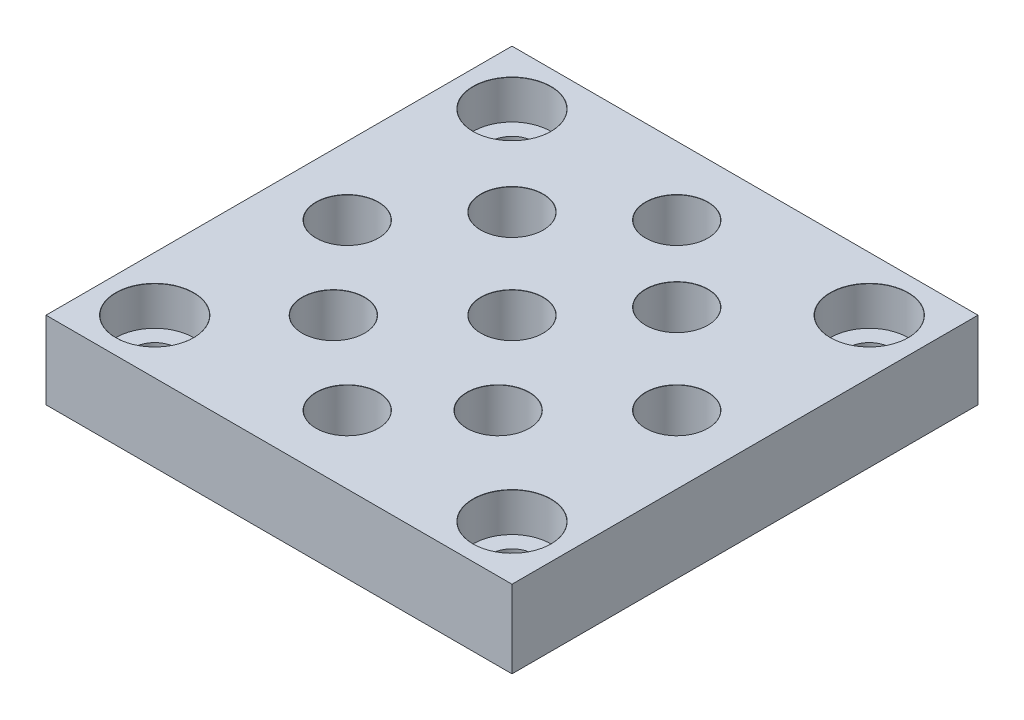
ISO-10303-21;
HEADER;
FILE_DESCRIPTION(('STEP AP214'),'2;1');
FILE_NAME('part.step','',(''),(''),'','','');
FILE_SCHEMA(('AUTOMOTIVE_DESIGN { 1 0 10303 214 1 1 1 1 }'));
ENDSEC;
DATA;
#1=APPLICATION_CONTEXT('core data for automotive mechanical design processes');
#2=APPLICATION_PROTOCOL_DEFINITION('international standard','automotive_design',2000,#1);
#3=PRODUCT_CONTEXT('',#1,'mechanical');
#4=PRODUCT('Part','Part','',(#3));
#5=PRODUCT_RELATED_PRODUCT_CATEGORY('part','',(#4));
#6=PRODUCT_DEFINITION_FORMATION('','',#4);
#7=PRODUCT_DEFINITION_CONTEXT('part definition',#1,'design');
#8=PRODUCT_DEFINITION('design','',#6,#7);
#9=PRODUCT_DEFINITION_SHAPE('','',#8);
#10=(LENGTH_UNIT() NAMED_UNIT(*) SI_UNIT(.MILLI.,.METRE.));
#11=(NAMED_UNIT(*) PLANE_ANGLE_UNIT() SI_UNIT($,.RADIAN.));
#12=(NAMED_UNIT(*) SI_UNIT($,.STERADIAN.) SOLID_ANGLE_UNIT());
#13=UNCERTAINTY_MEASURE_WITH_UNIT(LENGTH_MEASURE(1.E-05),#10,'distance_accuracy_value','');
#14=(GEOMETRIC_REPRESENTATION_CONTEXT(3) GLOBAL_UNCERTAINTY_ASSIGNED_CONTEXT((#13)) GLOBAL_UNIT_ASSIGNED_CONTEXT((#10,
#11,#12)) REPRESENTATION_CONTEXT('',''));
#15=CARTESIAN_POINT('',(0.,0.,0.));
#16=DIRECTION('',(0.,0.,1.));
#17=DIRECTION('',(1.,0.,0.));
#18=AXIS2_PLACEMENT_3D('',#15,#16,#17);
#19=CARTESIAN_POINT('',(0.,10.,0.));
#20=DIRECTION('',(0.,-1.,0.));
#21=DIRECTION('',(0.,0.,-1.));
#22=AXIS2_PLACEMENT_3D('',#19,#20,#21);
#23=PLANE('',#22);
#24=CARTESIAN_POINT('',(-21.2132034355964,10.,0.));
#25=DIRECTION('',(0.,1.,0.));
#26=DIRECTION('',(0.,0.,1.));
#27=AXIS2_PLACEMENT_3D('',#24,#25,#26);
#28=CIRCLE('',#27,4.025);
#29=CARTESIAN_POINT('',(-21.2132034355964,10.,4.025));
#30=VERTEX_POINT('',#29);
#31=EDGE_CURVE('E630',#30,#30,#28,.T.);
#32=ORIENTED_EDGE('',*,*,#31,.F.);
#33=EDGE_LOOP('',(#32));
#34=FACE_BOUND('',#33,.T.);
#35=CARTESIAN_POINT('',(0.,10.,0.));
#36=DIRECTION('',(0.,1.,0.));
#37=DIRECTION('',(0.,0.,1.));
#38=AXIS2_PLACEMENT_3D('',#35,#36,#37);
#39=CIRCLE('',#38,4.025);
#40=CARTESIAN_POINT('',(0.,10.,4.025));
#41=VERTEX_POINT('',#40);
#42=EDGE_CURVE('E176',#41,#41,#39,.T.);
#43=ORIENTED_EDGE('',*,*,#42,.F.);
#44=EDGE_LOOP('',(#43));
#45=FACE_BOUND('',#44,.T.);
#46=CARTESIAN_POINT('',(-11.5,10.,-11.5));
#47=DIRECTION('',(0.,1.,0.));
#48=DIRECTION('',(0.,0.,1.));
#49=AXIS2_PLACEMENT_3D('',#46,#47,#48);
#50=CIRCLE('',#49,4.025);
#51=CARTESIAN_POINT('',(-11.5,10.,-7.475));
#52=VERTEX_POINT('',#51);
#53=EDGE_CURVE('E164',#52,#52,#50,.T.);
#54=ORIENTED_EDGE('',*,*,#53,.F.);
#55=EDGE_LOOP('',(#54));
#56=FACE_BOUND('',#55,.T.);
#57=CARTESIAN_POINT('',(0.,10.,-21.2132034355964));
#58=DIRECTION('',(0.,1.,0.));
#59=DIRECTION('',(0.,0.,1.));
#60=AXIS2_PLACEMENT_3D('',#57,#58,#59);
#61=CIRCLE('',#60,4.025);
#62=CARTESIAN_POINT('',(0.,10.,-17.1882034355964));
#63=VERTEX_POINT('',#62);
#64=EDGE_CURVE('E156',#63,#63,#61,.T.);
#65=ORIENTED_EDGE('',*,*,#64,.F.);
#66=EDGE_LOOP('',(#65));
#67=FACE_BOUND('',#66,.T.);
#68=CARTESIAN_POINT('',(-11.5,10.,11.5));
#69=DIRECTION('',(0.,1.,0.));
#70=DIRECTION('',(0.,0.,1.));
#71=AXIS2_PLACEMENT_3D('',#68,#69,#70);
#72=CIRCLE('',#71,4.025);
#73=CARTESIAN_POINT('',(-11.5,10.,15.525));
#74=VERTEX_POINT('',#73);
#75=EDGE_CURVE('E151',#74,#74,#72,.T.);
#76=ORIENTED_EDGE('',*,*,#75,.F.);
#77=EDGE_LOOP('',(#76));
#78=FACE_BOUND('',#77,.T.);
#79=CARTESIAN_POINT('',(9.71320343559641,10.,11.5));
#80=DIRECTION('',(0.,1.,0.));
#81=DIRECTION('',(0.,0.,1.));
#82=AXIS2_PLACEMENT_3D('',#79,#80,#81);
#83=CIRCLE('',#82,4.025);
#84=CARTESIAN_POINT('',(9.71320343559641,10.,15.525));
#85=VERTEX_POINT('',#84);
#86=EDGE_CURVE('E148',#85,#85,#83,.T.);
#87=ORIENTED_EDGE('',*,*,#86,.F.);
#88=EDGE_LOOP('',(#87));
#89=FACE_BOUND('',#88,.T.);
#90=CARTESIAN_POINT('',(0.,10.,21.2132034355964));
#91=DIRECTION('',(0.,1.,0.));
#92=DIRECTION('',(0.,0.,1.));
#93=AXIS2_PLACEMENT_3D('',#90,#91,#92);
#94=CIRCLE('',#93,4.025);
#95=CARTESIAN_POINT('',(0.,10.,25.2382034355964));
#96=VERTEX_POINT('',#95);
#97=EDGE_CURVE('E143',#96,#96,#94,.T.);
#98=ORIENTED_EDGE('',*,*,#97,.F.);
#99=EDGE_LOOP('',(#98));
#100=FACE_BOUND('',#99,.T.);
#101=CARTESIAN_POINT('',(-23.,10.,-23.));
#102=DIRECTION('',(0.,1.,0.));
#103=DIRECTION('',(0.,0.,1.));
#104=AXIS2_PLACEMENT_3D('',#101,#102,#103);
#105=CIRCLE('',#104,5.025);
#106=CARTESIAN_POINT('',(-23.,10.,-17.975));
#107=VERTEX_POINT('',#106);
#108=EDGE_CURVE('E136',#107,#107,#105,.T.);
#109=ORIENTED_EDGE('',*,*,#108,.F.);
#110=EDGE_LOOP('',(#109));
#111=FACE_BOUND('',#110,.T.);
#112=CARTESIAN_POINT('',(23.,10.,-23.));
#113=DIRECTION('',(0.,1.,0.));
#114=DIRECTION('',(0.,0.,1.));
#115=AXIS2_PLACEMENT_3D('',#112,#113,#114);
#116=CIRCLE('',#115,5.025);
#117=CARTESIAN_POINT('',(23.,10.,-17.975));
#118=VERTEX_POINT('',#117);
#119=EDGE_CURVE('E134',#118,#118,#116,.T.);
#120=ORIENTED_EDGE('',*,*,#119,.F.);
#121=EDGE_LOOP('',(#120));
#122=FACE_BOUND('',#121,.T.);
#123=CARTESIAN_POINT('',(23.,10.,23.));
#124=DIRECTION('',(0.,1.,0.));
#125=DIRECTION('',(0.,0.,1.));
#126=AXIS2_PLACEMENT_3D('',#123,#124,#125);
#127=CIRCLE('',#126,5.025);
#128=CARTESIAN_POINT('',(23.,10.,28.025));
#129=VERTEX_POINT('',#128);
#130=EDGE_CURVE('E127',#129,#129,#127,.T.);
#131=ORIENTED_EDGE('',*,*,#130,.F.);
#132=EDGE_LOOP('',(#131));
#133=FACE_BOUND('',#132,.T.);
#134=CARTESIAN_POINT('',(-23.,10.,23.));
#135=DIRECTION('',(0.,1.,0.));
#136=DIRECTION('',(0.,0.,1.));
#137=AXIS2_PLACEMENT_3D('',#134,#135,#136);
#138=CIRCLE('',#137,5.025);
#139=CARTESIAN_POINT('',(-23.,10.,28.025));
#140=VERTEX_POINT('',#139);
#141=EDGE_CURVE('E121',#140,#140,#138,.T.);
#142=ORIENTED_EDGE('',*,*,#141,.F.);
#143=EDGE_LOOP('',(#142));
#144=FACE_BOUND('',#143,.T.);
#145=DIRECTION('',(0.,0.,1.));
#146=VECTOR('',#145,1.);
#147=CARTESIAN_POINT('',(-30.,10.,-30.));
#148=LINE('',#147,#146);
#149=CARTESIAN_POINT('',(-30.,10.,-30.));
#150=VERTEX_POINT('',#149);
#151=CARTESIAN_POINT('',(-30.,10.,30.));
#152=VERTEX_POINT('',#151);
#153=EDGE_CURVE('E91',#150,#152,#148,.T.);
#154=ORIENTED_EDGE('',*,*,#153,.T.);
#155=DIRECTION('',(1.,0.,0.));
#156=VECTOR('',#155,1.);
#157=CARTESIAN_POINT('',(30.,10.,30.));
#158=LINE('',#157,#156);
#159=CARTESIAN_POINT('',(30.,10.,30.));
#160=VERTEX_POINT('',#159);
#161=EDGE_CURVE('E86',#152,#160,#158,.T.);
#162=ORIENTED_EDGE('',*,*,#161,.T.);
#163=DIRECTION('',(0.,0.,-1.));
#164=VECTOR('',#163,1.);
#165=CARTESIAN_POINT('',(30.,10.,-30.));
#166=LINE('',#165,#164);
#167=CARTESIAN_POINT('',(30.,10.,-30.));
#168=VERTEX_POINT('',#167);
#169=EDGE_CURVE('E93',#160,#168,#166,.T.);
#170=ORIENTED_EDGE('',*,*,#169,.T.);
#171=DIRECTION('',(-1.,0.,0.));
#172=VECTOR('',#171,1.);
#173=CARTESIAN_POINT('',(30.,10.,-30.));
#174=LINE('',#173,#172);
#175=EDGE_CURVE('E59',#168,#150,#174,.T.);
#176=ORIENTED_EDGE('',*,*,#175,.T.);
#177=EDGE_LOOP('',(#154,#162,#170,#176));
#178=FACE_BOUND('',#177,.T.);
#179=CARTESIAN_POINT('',(9.71320343559641,10.,-11.5));
#180=DIRECTION('',(0.,1.,0.));
#181=DIRECTION('',(0.,0.,1.));
#182=AXIS2_PLACEMENT_3D('',#179,#180,#181);
#183=CIRCLE('',#182,4.025);
#184=CARTESIAN_POINT('',(9.71320343559641,10.,-7.475));
#185=VERTEX_POINT('',#184);
#186=EDGE_CURVE('E161',#185,#185,#183,.T.);
#187=ORIENTED_EDGE('',*,*,#186,.F.);
#188=EDGE_LOOP('',(#187));
#189=FACE_BOUND('',#188,.T.);
#190=CARTESIAN_POINT('',(21.2132034355964,10.,0.));
#191=DIRECTION('',(0.,1.,0.));
#192=DIRECTION('',(0.,0.,1.));
#193=AXIS2_PLACEMENT_3D('',#190,#191,#192);
#194=CIRCLE('',#193,4.025);
#195=CARTESIAN_POINT('',(21.2132034355964,10.,4.025));
#196=VERTEX_POINT('',#195);
#197=EDGE_CURVE('E166',#196,#196,#194,.T.);
#198=ORIENTED_EDGE('',*,*,#197,.F.);
#199=EDGE_LOOP('',(#198));
#200=FACE_BOUND('',#199,.T.);
#201=ADVANCED_FACE('F39',(#34,#45,#56,#67,#78,#89,#100,#111,#122,#133,#144,#178,#189,#200),#23,.F.);
#202=CARTESIAN_POINT('',(-30.,10.,-30.));
#203=DIRECTION('',(1.,0.,0.));
#204=DIRECTION('',(0.,0.,-1.));
#205=AXIS2_PLACEMENT_3D('',#202,#203,#204);
#206=PLANE('',#205);
#207=DIRECTION('',(0.,0.,1.));
#208=VECTOR('',#207,1.);
#209=CARTESIAN_POINT('',(-30.,0.,-30.));
#210=LINE('',#209,#208);
#211=CARTESIAN_POINT('',(-30.,0.,-30.));
#212=VERTEX_POINT('',#211);
#213=CARTESIAN_POINT('',(-30.,0.,30.));
#214=VERTEX_POINT('',#213);
#215=EDGE_CURVE('E106',#212,#214,#210,.T.);
#216=ORIENTED_EDGE('',*,*,#215,.T.);
#217=DIRECTION('',(0.,-1.,0.));
#218=VECTOR('',#217,1.);
#219=CARTESIAN_POINT('',(-30.,10.,30.));
#220=LINE('',#219,#218);
#221=EDGE_CURVE('E11',#152,#214,#220,.T.);
#222=ORIENTED_EDGE('',*,*,#221,.F.);
#223=ORIENTED_EDGE('',*,*,#153,.F.);
#224=DIRECTION('',(0.,-1.,0.));
#225=VECTOR('',#224,1.);
#226=CARTESIAN_POINT('',(-30.,10.,-30.));
#227=LINE('',#226,#225);
#228=EDGE_CURVE('E105',#150,#212,#227,.T.);
#229=ORIENTED_EDGE('',*,*,#228,.T.);
#230=EDGE_LOOP('',(#216,#222,#223,#229));
#231=FACE_BOUND('',#230,.T.);
#232=ADVANCED_FACE('F41',(#231),#206,.F.);
#233=CARTESIAN_POINT('',(30.,10.,30.));
#234=DIRECTION('',(0.,0.,-1.));
#235=DIRECTION('',(-1.,0.,0.));
#236=AXIS2_PLACEMENT_3D('',#233,#234,#235);
#237=PLANE('',#236);
#238=DIRECTION('',(1.,0.,0.));
#239=VECTOR('',#238,1.);
#240=CARTESIAN_POINT('',(30.,0.,30.));
#241=LINE('',#240,#239);
#242=CARTESIAN_POINT('',(30.,0.,30.));
#243=VERTEX_POINT('',#242);
#244=EDGE_CURVE('E100',#214,#243,#241,.T.);
#245=ORIENTED_EDGE('',*,*,#244,.T.);
#246=DIRECTION('',(0.,-1.,0.));
#247=VECTOR('',#246,1.);
#248=CARTESIAN_POINT('',(30.,10.,30.));
#249=LINE('',#248,#247);
#250=EDGE_CURVE('E47',#160,#243,#249,.T.);
#251=ORIENTED_EDGE('',*,*,#250,.F.);
#252=ORIENTED_EDGE('',*,*,#161,.F.);
#253=ORIENTED_EDGE('',*,*,#221,.T.);
#254=EDGE_LOOP('',(#245,#251,#252,#253));
#255=FACE_BOUND('',#254,.T.);
#256=ADVANCED_FACE('F96',(#255),#237,.F.);
#257=CARTESIAN_POINT('',(30.,10.,-30.));
#258=DIRECTION('',(-1.,0.,0.));
#259=DIRECTION('',(0.,0.,1.));
#260=AXIS2_PLACEMENT_3D('',#257,#258,#259);
#261=PLANE('',#260);
#262=DIRECTION('',(0.,0.,-1.));
#263=VECTOR('',#262,1.);
#264=CARTESIAN_POINT('',(30.,0.,-30.));
#265=LINE('',#264,#263);
#266=CARTESIAN_POINT('',(30.,0.,-30.));
#267=VERTEX_POINT('',#266);
#268=EDGE_CURVE('E73',#243,#267,#265,.T.);
#269=ORIENTED_EDGE('',*,*,#268,.T.);
#270=DIRECTION('',(0.,-1.,0.));
#271=VECTOR('',#270,1.);
#272=CARTESIAN_POINT('',(30.,10.,-30.));
#273=LINE('',#272,#271);
#274=EDGE_CURVE('E98',#168,#267,#273,.T.);
#275=ORIENTED_EDGE('',*,*,#274,.F.);
#276=ORIENTED_EDGE('',*,*,#169,.F.);
#277=ORIENTED_EDGE('',*,*,#250,.T.);
#278=EDGE_LOOP('',(#269,#275,#276,#277));
#279=FACE_BOUND('',#278,.T.);
#280=ADVANCED_FACE('F99',(#279),#261,.F.);
#281=CARTESIAN_POINT('',(30.,10.,-30.));
#282=DIRECTION('',(0.,0.,1.));
#283=DIRECTION('',(1.,0.,0.));
#284=AXIS2_PLACEMENT_3D('',#281,#282,#283);
#285=PLANE('',#284);
#286=DIRECTION('',(-1.,0.,0.));
#287=VECTOR('',#286,1.);
#288=CARTESIAN_POINT('',(30.,0.,-30.));
#289=LINE('',#288,#287);
#290=EDGE_CURVE('E81',#267,#212,#289,.T.);
#291=ORIENTED_EDGE('',*,*,#290,.T.);
#292=ORIENTED_EDGE('',*,*,#228,.F.);
#293=ORIENTED_EDGE('',*,*,#175,.F.);
#294=ORIENTED_EDGE('',*,*,#274,.T.);
#295=EDGE_LOOP('',(#291,#292,#293,#294));
#296=FACE_BOUND('',#295,.T.);
#297=ADVANCED_FACE('F290',(#296),#285,.F.);
#298=CARTESIAN_POINT('',(0.,0.,0.));
#299=DIRECTION('',(0.,-1.,0.));
#300=DIRECTION('',(0.,0.,-1.));
#301=AXIS2_PLACEMENT_3D('',#298,#299,#300);
#302=PLANE('',#301);
#303=CARTESIAN_POINT('',(-21.2132034355964,0.,0.));
#304=DIRECTION('',(0.,-1.,0.));
#305=DIRECTION('',(0.,0.,-1.));
#306=AXIS2_PLACEMENT_3D('',#303,#304,#305);
#307=CIRCLE('',#306,3.99999999999999);
#308=CARTESIAN_POINT('',(-21.2132034355964,0.,-4.));
#309=VERTEX_POINT('',#308);
#310=EDGE_CURVE('E43',#309,#309,#307,.T.);
#311=ORIENTED_EDGE('',*,*,#310,.F.);
#312=EDGE_LOOP('',(#311));
#313=FACE_BOUND('',#312,.T.);
#314=CARTESIAN_POINT('',(0.,0.,0.));
#315=DIRECTION('',(0.,-1.,0.));
#316=DIRECTION('',(0.,0.,-1.));
#317=AXIS2_PLACEMENT_3D('',#314,#315,#316);
#318=CIRCLE('',#317,3.99999999999999);
#319=CARTESIAN_POINT('',(0.,0.,-3.99999999999999));
#320=VERTEX_POINT('',#319);
#321=EDGE_CURVE('E170',#320,#320,#318,.T.);
#322=ORIENTED_EDGE('',*,*,#321,.F.);
#323=EDGE_LOOP('',(#322));
#324=FACE_BOUND('',#323,.T.);
#325=CARTESIAN_POINT('',(21.2132034355964,0.,0.));
#326=DIRECTION('',(0.,-1.,0.));
#327=DIRECTION('',(0.,0.,-1.));
#328=AXIS2_PLACEMENT_3D('',#325,#326,#327);
#329=CIRCLE('',#328,3.99999999999999);
#330=CARTESIAN_POINT('',(21.2132034355964,0.,-3.99999999999999));
#331=VERTEX_POINT('',#330);
#332=EDGE_CURVE('E162',#331,#331,#329,.T.);
#333=ORIENTED_EDGE('',*,*,#332,.F.);
#334=EDGE_LOOP('',(#333));
#335=FACE_BOUND('',#334,.T.);
#336=CARTESIAN_POINT('',(-11.5,0.,-11.5));
#337=DIRECTION('',(0.,-1.,0.));
#338=DIRECTION('',(0.,0.,-1.));
#339=AXIS2_PLACEMENT_3D('',#336,#337,#338);
#340=CIRCLE('',#339,3.99999999999999);
#341=CARTESIAN_POINT('',(-11.5,0.,-15.5));
#342=VERTEX_POINT('',#341);
#343=EDGE_CURVE('E158',#342,#342,#340,.T.);
#344=ORIENTED_EDGE('',*,*,#343,.F.);
#345=EDGE_LOOP('',(#344));
#346=FACE_BOUND('',#345,.T.);
#347=CARTESIAN_POINT('',(9.71320343559641,0.,-11.5));
#348=DIRECTION('',(0.,-1.,0.));
#349=DIRECTION('',(0.,0.,-1.));
#350=AXIS2_PLACEMENT_3D('',#347,#348,#349);
#351=CIRCLE('',#350,3.99999999999999);
#352=CARTESIAN_POINT('',(9.71320343559641,0.,-15.5));
#353=VERTEX_POINT('',#352);
#354=EDGE_CURVE('E153',#353,#353,#351,.T.);
#355=ORIENTED_EDGE('',*,*,#354,.F.);
#356=EDGE_LOOP('',(#355));
#357=FACE_BOUND('',#356,.T.);
#358=CARTESIAN_POINT('',(0.,0.,-21.2132034355964));
#359=DIRECTION('',(0.,-1.,0.));
#360=DIRECTION('',(0.,0.,-1.));
#361=AXIS2_PLACEMENT_3D('',#358,#359,#360);
#362=CIRCLE('',#361,3.99999999999999);
#363=CARTESIAN_POINT('',(0.,0.,-25.2132034355964));
#364=VERTEX_POINT('',#363);
#365=EDGE_CURVE('E146',#364,#364,#362,.T.);
#366=ORIENTED_EDGE('',*,*,#365,.F.);
#367=EDGE_LOOP('',(#366));
#368=FACE_BOUND('',#367,.T.);
#369=CARTESIAN_POINT('',(-11.5,0.,11.5));
#370=DIRECTION('',(0.,-1.,0.));
#371=DIRECTION('',(0.,0.,-1.));
#372=AXIS2_PLACEMENT_3D('',#369,#370,#371);
#373=CIRCLE('',#372,3.99999999999999);
#374=CARTESIAN_POINT('',(-11.5,0.,7.5));
#375=VERTEX_POINT('',#374);
#376=EDGE_CURVE('E141',#375,#375,#373,.T.);
#377=ORIENTED_EDGE('',*,*,#376,.F.);
#378=EDGE_LOOP('',(#377));
#379=FACE_BOUND('',#378,.T.);
#380=CARTESIAN_POINT('',(9.71320343559641,0.,11.5));
#381=DIRECTION('',(0.,-1.,0.));
#382=DIRECTION('',(0.,0.,-1.));
#383=AXIS2_PLACEMENT_3D('',#380,#381,#382);
#384=CIRCLE('',#383,3.99999999999999);
#385=CARTESIAN_POINT('',(9.71320343559641,0.,7.50000000000001));
#386=VERTEX_POINT('',#385);
#387=EDGE_CURVE('E138',#386,#386,#384,.T.);
#388=ORIENTED_EDGE('',*,*,#387,.F.);
#389=EDGE_LOOP('',(#388));
#390=FACE_BOUND('',#389,.T.);
#391=CARTESIAN_POINT('',(0.,0.,21.2132034355964));
#392=DIRECTION('',(0.,-1.,0.));
#393=DIRECTION('',(0.,0.,-1.));
#394=AXIS2_PLACEMENT_3D('',#391,#392,#393);
#395=CIRCLE('',#394,3.99999999999999);
#396=CARTESIAN_POINT('',(0.,0.,17.2132034355964));
#397=VERTEX_POINT('',#396);
#398=EDGE_CURVE('E135',#397,#397,#395,.T.);
#399=ORIENTED_EDGE('',*,*,#398,.F.);
#400=EDGE_LOOP('',(#399));
#401=FACE_BOUND('',#400,.T.);
#402=CARTESIAN_POINT('',(-23.,0.,-23.));
#403=DIRECTION('',(0.,-1.,0.));
#404=DIRECTION('',(0.,0.,-1.));
#405=AXIS2_PLACEMENT_3D('',#402,#403,#404);
#406=CIRCLE('',#405,2.74999999999999);
#407=CARTESIAN_POINT('',(-23.,0.,-25.75));
#408=VERTEX_POINT('',#407);
#409=EDGE_CURVE('E126',#408,#408,#406,.T.);
#410=ORIENTED_EDGE('',*,*,#409,.F.);
#411=EDGE_LOOP('',(#410));
#412=FACE_BOUND('',#411,.T.);
#413=CARTESIAN_POINT('',(23.,0.,-23.));
#414=DIRECTION('',(0.,-1.,0.));
#415=DIRECTION('',(0.,0.,-1.));
#416=AXIS2_PLACEMENT_3D('',#413,#414,#415);
#417=CIRCLE('',#416,2.74999999999999);
#418=CARTESIAN_POINT('',(23.,0.,-25.75));
#419=VERTEX_POINT('',#418);
#420=EDGE_CURVE('E123',#419,#419,#417,.T.);
#421=ORIENTED_EDGE('',*,*,#420,.F.);
#422=EDGE_LOOP('',(#421));
#423=FACE_BOUND('',#422,.T.);
#424=CARTESIAN_POINT('',(23.,0.,23.));
#425=DIRECTION('',(0.,-1.,0.));
#426=DIRECTION('',(0.,0.,-1.));
#427=AXIS2_PLACEMENT_3D('',#424,#425,#426);
#428=CIRCLE('',#427,2.74999999999999);
#429=CARTESIAN_POINT('',(23.,0.,20.25));
#430=VERTEX_POINT('',#429);
#431=EDGE_CURVE('E120',#430,#430,#428,.T.);
#432=ORIENTED_EDGE('',*,*,#431,.F.);
#433=EDGE_LOOP('',(#432));
#434=FACE_BOUND('',#433,.T.);
#435=CARTESIAN_POINT('',(-23.,0.,23.));
#436=DIRECTION('',(0.,-1.,0.));
#437=DIRECTION('',(0.,0.,-1.));
#438=AXIS2_PLACEMENT_3D('',#435,#436,#437);
#439=CIRCLE('',#438,2.74999999999999);
#440=CARTESIAN_POINT('',(-23.,0.,20.25));
#441=VERTEX_POINT('',#440);
#442=EDGE_CURVE('E108',#441,#441,#439,.T.);
#443=ORIENTED_EDGE('',*,*,#442,.F.);
#444=EDGE_LOOP('',(#443));
#445=FACE_BOUND('',#444,.T.);
#446=ORIENTED_EDGE('',*,*,#215,.F.);
#447=ORIENTED_EDGE('',*,*,#290,.F.);
#448=ORIENTED_EDGE('',*,*,#268,.F.);
#449=ORIENTED_EDGE('',*,*,#244,.F.);
#450=EDGE_LOOP('',(#446,#447,#448,#449));
#451=FACE_BOUND('',#450,.T.);
#452=ADVANCED_FACE('F282',(#313,#324,#335,#346,#357,#368,#379,#390,#401,#412,#423,#434,#445,
#451),#302,.T.);
#453=CARTESIAN_POINT('',(-23.,10.,23.));
#454=DIRECTION('',(0.,1.,0.));
#455=DIRECTION('',(0.,0.,1.));
#456=AXIS2_PLACEMENT_3D('',#453,#454,#455);
#457=CYLINDRICAL_SURFACE('',#456,2.74999999999999);
#458=ORIENTED_EDGE('',*,*,#442,.T.);
#459=EDGE_LOOP('',(#458));
#460=FACE_BOUND('',#459,.T.);
#461=CARTESIAN_POINT('',(-23.,5.,23.));
#462=DIRECTION('',(0.,1.,0.));
#463=DIRECTION('',(0.,0.,1.));
#464=AXIS2_PLACEMENT_3D('',#461,#462,#463);
#465=CIRCLE('',#464,2.75);
#466=CARTESIAN_POINT('',(-23.,5.,25.75));
#467=VERTEX_POINT('',#466);
#468=EDGE_CURVE('E116',#467,#467,#465,.T.);
#469=ORIENTED_EDGE('',*,*,#468,.T.);
#470=EDGE_LOOP('',(#469));
#471=FACE_BOUND('',#470,.T.);
#472=ADVANCED_FACE('F253',(#460,#471),#457,.F.);
#473=CARTESIAN_POINT('',(-20.25,5.,23.));
#474=DIRECTION('',(0.,-1.,0.));
#475=DIRECTION('',(0.,0.,-1.));
#476=AXIS2_PLACEMENT_3D('',#473,#474,#475);
#477=PLANE('',#476);
#478=ORIENTED_EDGE('',*,*,#468,.F.);
#479=EDGE_LOOP('',(#478));
#480=FACE_BOUND('',#479,.T.);
#481=CARTESIAN_POINT('',(-23.,5.,23.));
#482=DIRECTION('',(0.,1.,0.));
#483=DIRECTION('',(0.,0.,1.));
#484=AXIS2_PLACEMENT_3D('',#481,#482,#483);
#485=CIRCLE('',#484,5.);
#486=CARTESIAN_POINT('',(-23.,5.,28.));
#487=VERTEX_POINT('',#486);
#488=EDGE_CURVE('E242',#487,#487,#485,.T.);
#489=ORIENTED_EDGE('',*,*,#488,.T.);
#490=EDGE_LOOP('',(#489));
#491=FACE_BOUND('',#490,.T.);
#492=ADVANCED_FACE('F251',(#480,#491),#477,.F.);
#493=CARTESIAN_POINT('',(-23.,10.,23.));
#494=DIRECTION('',(0.,1.,0.));
#495=DIRECTION('',(0.,0.,1.));
#496=AXIS2_PLACEMENT_3D('',#493,#494,#495);
#497=CYLINDRICAL_SURFACE('',#496,5.);
#498=ORIENTED_EDGE('',*,*,#488,.F.);
#499=EDGE_LOOP('',(#498));
#500=FACE_BOUND('',#499,.T.);
#501=CARTESIAN_POINT('',(-23.,9.97902250922057,23.));
#502=DIRECTION('',(0.,1.,0.));
#503=DIRECTION('',(0.,0.,1.));
#504=AXIS2_PLACEMENT_3D('',#501,#502,#503);
#505=CIRCLE('',#504,5.);
#506=CARTESIAN_POINT('',(-23.,9.97902250922057,28.));
#507=VERTEX_POINT('',#506);
#508=EDGE_CURVE('E241',#507,#507,#505,.T.);
#509=ORIENTED_EDGE('',*,*,#508,.T.);
#510=EDGE_LOOP('',(#509));
#511=FACE_BOUND('',#510,.T.);
#512=ADVANCED_FACE('F258',(#500,#511),#497,.F.);
#513=CARTESIAN_POINT('',(-23.,10.,23.));
#514=DIRECTION('',(0.,1.,0.));
#515=DIRECTION('',(0.,0.,1.));
#516=AXIS2_PLACEMENT_3D('',#513,#514,#515);
#517=CONICAL_SURFACE('',#516,5.025,0.872664625997159);
#518=ORIENTED_EDGE('',*,*,#508,.F.);
#519=EDGE_LOOP('',(#518));
#520=FACE_BOUND('',#519,.T.);
#521=ORIENTED_EDGE('',*,*,#141,.T.);
#522=EDGE_LOOP('',(#521));
#523=FACE_BOUND('',#522,.T.);
#524=ADVANCED_FACE('F265',(#520,#523),#517,.F.);
#525=CARTESIAN_POINT('',(23.,10.,23.));
#526=DIRECTION('',(0.,1.,0.));
#527=DIRECTION('',(0.,0.,1.));
#528=AXIS2_PLACEMENT_3D('',#525,#526,#527);
#529=CYLINDRICAL_SURFACE('',#528,2.74999999999999);
#530=ORIENTED_EDGE('',*,*,#431,.T.);
#531=EDGE_LOOP('',(#530));
#532=FACE_BOUND('',#531,.T.);
#533=CARTESIAN_POINT('',(23.,5.,23.));
#534=DIRECTION('',(0.,1.,0.));
#535=DIRECTION('',(0.,0.,1.));
#536=AXIS2_PLACEMENT_3D('',#533,#534,#535);
#537=CIRCLE('',#536,2.75);
#538=CARTESIAN_POINT('',(23.,5.,25.75));
#539=VERTEX_POINT('',#538);
#540=EDGE_CURVE('E125',#539,#539,#537,.T.);
#541=ORIENTED_EDGE('',*,*,#540,.T.);
#542=EDGE_LOOP('',(#541));
#543=FACE_BOUND('',#542,.T.);
#544=ADVANCED_FACE('F268',(#532,#543),#529,.F.);
#545=CARTESIAN_POINT('',(25.75,5.,23.));
#546=DIRECTION('',(0.,-1.,0.));
#547=DIRECTION('',(0.,0.,-1.));
#548=AXIS2_PLACEMENT_3D('',#545,#546,#547);
#549=PLANE('',#548);
#550=ORIENTED_EDGE('',*,*,#540,.F.);
#551=EDGE_LOOP('',(#550));
#552=FACE_BOUND('',#551,.T.);
#553=CARTESIAN_POINT('',(23.,5.,23.));
#554=DIRECTION('',(0.,1.,0.));
#555=DIRECTION('',(0.,0.,1.));
#556=AXIS2_PLACEMENT_3D('',#553,#554,#555);
#557=CIRCLE('',#556,5.);
#558=CARTESIAN_POINT('',(23.,5.,28.));
#559=VERTEX_POINT('',#558);
#560=EDGE_CURVE('E234',#559,#559,#557,.T.);
#561=ORIENTED_EDGE('',*,*,#560,.T.);
#562=EDGE_LOOP('',(#561));
#563=FACE_BOUND('',#562,.T.);
#564=ADVANCED_FACE('F336',(#552,#563),#549,.F.);
#565=CARTESIAN_POINT('',(23.,10.,23.));
#566=DIRECTION('',(0.,1.,0.));
#567=DIRECTION('',(0.,0.,1.));
#568=AXIS2_PLACEMENT_3D('',#565,#566,#567);
#569=CYLINDRICAL_SURFACE('',#568,5.);
#570=ORIENTED_EDGE('',*,*,#560,.F.);
#571=EDGE_LOOP('',(#570));
#572=FACE_BOUND('',#571,.T.);
#573=CARTESIAN_POINT('',(23.,9.97902250922057,23.));
#574=DIRECTION('',(0.,1.,0.));
#575=DIRECTION('',(0.,0.,1.));
#576=AXIS2_PLACEMENT_3D('',#573,#574,#575);
#577=CIRCLE('',#576,5.);
#578=CARTESIAN_POINT('',(23.,9.97902250922057,28.));
#579=VERTEX_POINT('',#578);
#580=EDGE_CURVE('E235',#579,#579,#577,.T.);
#581=ORIENTED_EDGE('',*,*,#580,.T.);
#582=EDGE_LOOP('',(#581));
#583=FACE_BOUND('',#582,.T.);
#584=ADVANCED_FACE('F347',(#572,#583),#569,.F.);
#585=CARTESIAN_POINT('',(23.,10.,23.));
#586=DIRECTION('',(0.,1.,0.));
#587=DIRECTION('',(0.,0.,1.));
#588=AXIS2_PLACEMENT_3D('',#585,#586,#587);
#589=CONICAL_SURFACE('',#588,5.025,0.872664625997159);
#590=ORIENTED_EDGE('',*,*,#580,.F.);
#591=EDGE_LOOP('',(#590));
#592=FACE_BOUND('',#591,.T.);
#593=ORIENTED_EDGE('',*,*,#130,.T.);
#594=EDGE_LOOP('',(#593));
#595=FACE_BOUND('',#594,.T.);
#596=ADVANCED_FACE('F352',(#592,#595),#589,.F.);
#597=CARTESIAN_POINT('',(23.,10.,-23.));
#598=DIRECTION('',(0.,1.,0.));
#599=DIRECTION('',(0.,0.,1.));
#600=AXIS2_PLACEMENT_3D('',#597,#598,#599);
#601=CYLINDRICAL_SURFACE('',#600,2.74999999999999);
#602=ORIENTED_EDGE('',*,*,#420,.T.);
#603=EDGE_LOOP('',(#602));
#604=FACE_BOUND('',#603,.T.);
#605=CARTESIAN_POINT('',(23.,5.,-23.));
#606=DIRECTION('',(0.,1.,0.));
#607=DIRECTION('',(0.,0.,1.));
#608=AXIS2_PLACEMENT_3D('',#605,#606,#607);
#609=CIRCLE('',#608,2.75);
#610=CARTESIAN_POINT('',(23.,5.,-20.25));
#611=VERTEX_POINT('',#610);
#612=EDGE_CURVE('E130',#611,#611,#609,.T.);
#613=ORIENTED_EDGE('',*,*,#612,.T.);
#614=EDGE_LOOP('',(#613));
#615=FACE_BOUND('',#614,.T.);
#616=ADVANCED_FACE('F365',(#604,#615),#601,.F.);
#617=CARTESIAN_POINT('',(25.75,5.,-23.));
#618=DIRECTION('',(0.,-1.,0.));
#619=DIRECTION('',(0.,0.,-1.));
#620=AXIS2_PLACEMENT_3D('',#617,#618,#619);
#621=PLANE('',#620);
#622=ORIENTED_EDGE('',*,*,#612,.F.);
#623=EDGE_LOOP('',(#622));
#624=FACE_BOUND('',#623,.T.);
#625=CARTESIAN_POINT('',(23.,5.,-23.));
#626=DIRECTION('',(0.,1.,0.));
#627=DIRECTION('',(0.,0.,1.));
#628=AXIS2_PLACEMENT_3D('',#625,#626,#627);
#629=CIRCLE('',#628,5.);
#630=CARTESIAN_POINT('',(23.,5.,-18.));
#631=VERTEX_POINT('',#630);
#632=EDGE_CURVE('E223',#631,#631,#629,.T.);
#633=ORIENTED_EDGE('',*,*,#632,.T.);
#634=EDGE_LOOP('',(#633));
#635=FACE_BOUND('',#634,.T.);
#636=ADVANCED_FACE('F373',(#624,#635),#621,.F.);
#637=CARTESIAN_POINT('',(23.,10.,-23.));
#638=DIRECTION('',(0.,1.,0.));
#639=DIRECTION('',(0.,0.,1.));
#640=AXIS2_PLACEMENT_3D('',#637,#638,#639);
#641=CYLINDRICAL_SURFACE('',#640,5.);
#642=ORIENTED_EDGE('',*,*,#632,.F.);
#643=EDGE_LOOP('',(#642));
#644=FACE_BOUND('',#643,.T.);
#645=CARTESIAN_POINT('',(23.,9.97902250922057,-23.));
#646=DIRECTION('',(0.,1.,0.));
#647=DIRECTION('',(0.,0.,1.));
#648=AXIS2_PLACEMENT_3D('',#645,#646,#647);
#649=CIRCLE('',#648,5.);
#650=CARTESIAN_POINT('',(23.,9.97902250922057,-18.));
#651=VERTEX_POINT('',#650);
#652=EDGE_CURVE('E225',#651,#651,#649,.T.);
#653=ORIENTED_EDGE('',*,*,#652,.T.);
#654=EDGE_LOOP('',(#653));
#655=FACE_BOUND('',#654,.T.);
#656=ADVANCED_FACE('F385',(#644,#655),#641,.F.);
#657=CARTESIAN_POINT('',(23.,10.,-23.));
#658=DIRECTION('',(0.,1.,0.));
#659=DIRECTION('',(0.,0.,1.));
#660=AXIS2_PLACEMENT_3D('',#657,#658,#659);
#661=CONICAL_SURFACE('',#660,5.025,0.872664625997159);
#662=ORIENTED_EDGE('',*,*,#652,.F.);
#663=EDGE_LOOP('',(#662));
#664=FACE_BOUND('',#663,.T.);
#665=ORIENTED_EDGE('',*,*,#119,.T.);
#666=EDGE_LOOP('',(#665));
#667=FACE_BOUND('',#666,.T.);
#668=ADVANCED_FACE('F394',(#664,#667),#661,.F.);
#669=CARTESIAN_POINT('',(-23.,10.,-23.));
#670=DIRECTION('',(0.,1.,0.));
#671=DIRECTION('',(0.,0.,1.));
#672=AXIS2_PLACEMENT_3D('',#669,#670,#671);
#673=CYLINDRICAL_SURFACE('',#672,2.74999999999999);
#674=ORIENTED_EDGE('',*,*,#409,.T.);
#675=EDGE_LOOP('',(#674));
#676=FACE_BOUND('',#675,.T.);
#677=CARTESIAN_POINT('',(-23.,5.,-23.));
#678=DIRECTION('',(0.,1.,0.));
#679=DIRECTION('',(0.,0.,1.));
#680=AXIS2_PLACEMENT_3D('',#677,#678,#679);
#681=CIRCLE('',#680,2.75);
#682=CARTESIAN_POINT('',(-23.,5.,-20.25));
#683=VERTEX_POINT('',#682);
#684=EDGE_CURVE('E131',#683,#683,#681,.T.);
#685=ORIENTED_EDGE('',*,*,#684,.T.);
#686=EDGE_LOOP('',(#685));
#687=FACE_BOUND('',#686,.T.);
#688=ADVANCED_FACE('F399',(#676,#687),#673,.F.);
#689=CARTESIAN_POINT('',(-20.25,5.,-23.));
#690=DIRECTION('',(0.,-1.,0.));
#691=DIRECTION('',(0.,0.,-1.));
#692=AXIS2_PLACEMENT_3D('',#689,#690,#691);
#693=PLANE('',#692);
#694=ORIENTED_EDGE('',*,*,#684,.F.);
#695=EDGE_LOOP('',(#694));
#696=FACE_BOUND('',#695,.T.);
#697=CARTESIAN_POINT('',(-23.,5.,-23.));
#698=DIRECTION('',(0.,1.,0.));
#699=DIRECTION('',(0.,0.,1.));
#700=AXIS2_PLACEMENT_3D('',#697,#698,#699);
#701=CIRCLE('',#700,5.);
#702=CARTESIAN_POINT('',(-23.,5.,-18.));
#703=VERTEX_POINT('',#702);
#704=EDGE_CURVE('E214',#703,#703,#701,.T.);
#705=ORIENTED_EDGE('',*,*,#704,.T.);
#706=EDGE_LOOP('',(#705));
#707=FACE_BOUND('',#706,.T.);
#708=ADVANCED_FACE('F408',(#696,#707),#693,.F.);
#709=CARTESIAN_POINT('',(-23.,10.,-23.));
#710=DIRECTION('',(0.,1.,0.));
#711=DIRECTION('',(0.,0.,1.));
#712=AXIS2_PLACEMENT_3D('',#709,#710,#711);
#713=CYLINDRICAL_SURFACE('',#712,5.);
#714=ORIENTED_EDGE('',*,*,#704,.F.);
#715=EDGE_LOOP('',(#714));
#716=FACE_BOUND('',#715,.T.);
#717=CARTESIAN_POINT('',(-23.,9.97902250922057,-23.));
#718=DIRECTION('',(0.,1.,0.));
#719=DIRECTION('',(0.,0.,1.));
#720=AXIS2_PLACEMENT_3D('',#717,#718,#719);
#721=CIRCLE('',#720,5.);
#722=CARTESIAN_POINT('',(-23.,9.97902250922057,-18.));
#723=VERTEX_POINT('',#722);
#724=EDGE_CURVE('E215',#723,#723,#721,.T.);
#725=ORIENTED_EDGE('',*,*,#724,.T.);
#726=EDGE_LOOP('',(#725));
#727=FACE_BOUND('',#726,.T.);
#728=ADVANCED_FACE('F416',(#716,#727),#713,.F.);
#729=CARTESIAN_POINT('',(-23.,10.,-23.));
#730=DIRECTION('',(0.,1.,0.));
#731=DIRECTION('',(0.,0.,1.));
#732=AXIS2_PLACEMENT_3D('',#729,#730,#731);
#733=CONICAL_SURFACE('',#732,5.025,0.872664625997159);
#734=ORIENTED_EDGE('',*,*,#724,.F.);
#735=EDGE_LOOP('',(#734));
#736=FACE_BOUND('',#735,.T.);
#737=ORIENTED_EDGE('',*,*,#108,.T.);
#738=EDGE_LOOP('',(#737));
#739=FACE_BOUND('',#738,.T.);
#740=ADVANCED_FACE('F426',(#736,#739),#733,.F.);
#741=CARTESIAN_POINT('',(0.,10.,21.2132034355964));
#742=DIRECTION('',(0.,1.,0.));
#743=DIRECTION('',(0.,0.,1.));
#744=AXIS2_PLACEMENT_3D('',#741,#742,#743);
#745=CYLINDRICAL_SURFACE('',#744,3.99999999999999);
#746=ORIENTED_EDGE('',*,*,#398,.T.);
#747=EDGE_LOOP('',(#746));
#748=FACE_BOUND('',#747,.T.);
#749=CARTESIAN_POINT('',(0.,9.97902250922057,21.2132034355964));
#750=DIRECTION('',(0.,1.,0.));
#751=DIRECTION('',(0.,0.,1.));
#752=AXIS2_PLACEMENT_3D('',#749,#750,#751);
#753=CIRCLE('',#752,4.);
#754=CARTESIAN_POINT('',(0.,9.97902250922057,25.2132034355964));
#755=VERTEX_POINT('',#754);
#756=EDGE_CURVE('E140',#755,#755,#753,.T.);
#757=ORIENTED_EDGE('',*,*,#756,.T.);
#758=EDGE_LOOP('',(#757));
#759=FACE_BOUND('',#758,.T.);
#760=ADVANCED_FACE('F432',(#748,#759),#745,.F.);
#761=CARTESIAN_POINT('',(0.,10.,21.2132034355964));
#762=DIRECTION('',(0.,1.,0.));
#763=DIRECTION('',(0.,0.,1.));
#764=AXIS2_PLACEMENT_3D('',#761,#762,#763);
#765=CONICAL_SURFACE('',#764,4.025,0.872664625997325);
#766=ORIENTED_EDGE('',*,*,#756,.F.);
#767=EDGE_LOOP('',(#766));
#768=FACE_BOUND('',#767,.T.);
#769=ORIENTED_EDGE('',*,*,#97,.T.);
#770=EDGE_LOOP('',(#769));
#771=FACE_BOUND('',#770,.T.);
#772=ADVANCED_FACE('F451',(#768,#771),#765,.F.);
#773=CARTESIAN_POINT('',(9.71320343559641,10.,11.5));
#774=DIRECTION('',(0.,1.,0.));
#775=DIRECTION('',(0.,0.,1.));
#776=AXIS2_PLACEMENT_3D('',#773,#774,#775);
#777=CYLINDRICAL_SURFACE('',#776,3.99999999999999);
#778=ORIENTED_EDGE('',*,*,#387,.T.);
#779=EDGE_LOOP('',(#778));
#780=FACE_BOUND('',#779,.T.);
#781=CARTESIAN_POINT('',(9.71320343559641,9.97902250922057,11.5));
#782=DIRECTION('',(0.,1.,0.));
#783=DIRECTION('',(0.,0.,1.));
#784=AXIS2_PLACEMENT_3D('',#781,#782,#783);
#785=CIRCLE('',#784,4.);
#786=CARTESIAN_POINT('',(9.71320343559641,9.97902250922057,15.5));
#787=VERTEX_POINT('',#786);
#788=EDGE_CURVE('E142',#787,#787,#785,.T.);
#789=ORIENTED_EDGE('',*,*,#788,.T.);
#790=EDGE_LOOP('',(#789));
#791=FACE_BOUND('',#790,.T.);
#792=ADVANCED_FACE('F464',(#780,#791),#777,.F.);
#793=CARTESIAN_POINT('',(9.71320343559641,10.,11.5));
#794=DIRECTION('',(0.,1.,0.));
#795=DIRECTION('',(0.,0.,1.));
#796=AXIS2_PLACEMENT_3D('',#793,#794,#795);
#797=CONICAL_SURFACE('',#796,4.025,0.872664625997308);
#798=ORIENTED_EDGE('',*,*,#788,.F.);
#799=EDGE_LOOP('',(#798));
#800=FACE_BOUND('',#799,.T.);
#801=ORIENTED_EDGE('',*,*,#86,.T.);
#802=EDGE_LOOP('',(#801));
#803=FACE_BOUND('',#802,.T.);
#804=ADVANCED_FACE('F473',(#800,#803),#797,.F.);
#805=CARTESIAN_POINT('',(-11.5,10.,11.5));
#806=DIRECTION('',(0.,1.,0.));
#807=DIRECTION('',(0.,0.,1.));
#808=AXIS2_PLACEMENT_3D('',#805,#806,#807);
#809=CYLINDRICAL_SURFACE('',#808,3.99999999999999);
#810=ORIENTED_EDGE('',*,*,#376,.T.);
#811=EDGE_LOOP('',(#810));
#812=FACE_BOUND('',#811,.T.);
#813=CARTESIAN_POINT('',(-11.5,9.97902250922057,11.5));
#814=DIRECTION('',(0.,1.,0.));
#815=DIRECTION('',(0.,0.,1.));
#816=AXIS2_PLACEMENT_3D('',#813,#814,#815);
#817=CIRCLE('',#816,4.);
#818=CARTESIAN_POINT('',(-11.5,9.97902250922057,15.5));
#819=VERTEX_POINT('',#818);
#820=EDGE_CURVE('E150',#819,#819,#817,.T.);
#821=ORIENTED_EDGE('',*,*,#820,.T.);
#822=EDGE_LOOP('',(#821));
#823=FACE_BOUND('',#822,.T.);
#824=ADVANCED_FACE('F481',(#812,#823),#809,.F.);
#825=CARTESIAN_POINT('',(-11.5,10.,11.5));
#826=DIRECTION('',(0.,1.,0.));
#827=DIRECTION('',(0.,0.,1.));
#828=AXIS2_PLACEMENT_3D('',#825,#826,#827);
#829=CONICAL_SURFACE('',#828,4.025,0.872664625997325);
#830=ORIENTED_EDGE('',*,*,#820,.F.);
#831=EDGE_LOOP('',(#830));
#832=FACE_BOUND('',#831,.T.);
#833=ORIENTED_EDGE('',*,*,#75,.T.);
#834=EDGE_LOOP('',(#833));
#835=FACE_BOUND('',#834,.T.);
#836=ADVANCED_FACE('F491',(#832,#835),#829,.F.);
#837=CARTESIAN_POINT('',(0.,10.,-21.2132034355964));
#838=DIRECTION('',(0.,1.,0.));
#839=DIRECTION('',(0.,0.,1.));
#840=AXIS2_PLACEMENT_3D('',#837,#838,#839);
#841=CYLINDRICAL_SURFACE('',#840,3.99999999999999);
#842=ORIENTED_EDGE('',*,*,#365,.T.);
#843=EDGE_LOOP('',(#842));
#844=FACE_BOUND('',#843,.T.);
#845=CARTESIAN_POINT('',(0.,9.97902250922057,-21.2132034355964));
#846=DIRECTION('',(0.,1.,0.));
#847=DIRECTION('',(0.,0.,1.));
#848=AXIS2_PLACEMENT_3D('',#845,#846,#847);
#849=CIRCLE('',#848,4.);
#850=CARTESIAN_POINT('',(0.,9.97902250922057,-17.2132034355964));
#851=VERTEX_POINT('',#850);
#852=EDGE_CURVE('E155',#851,#851,#849,.T.);
#853=ORIENTED_EDGE('',*,*,#852,.T.);
#854=EDGE_LOOP('',(#853));
#855=FACE_BOUND('',#854,.T.);
#856=ADVANCED_FACE('F504',(#844,#855),#841,.F.);
#857=CARTESIAN_POINT('',(0.,10.,-21.2132034355964));
#858=DIRECTION('',(0.,1.,0.));
#859=DIRECTION('',(0.,0.,1.));
#860=AXIS2_PLACEMENT_3D('',#857,#858,#859);
#861=CONICAL_SURFACE('',#860,4.025,0.872664625997325);
#862=ORIENTED_EDGE('',*,*,#852,.F.);
#863=EDGE_LOOP('',(#862));
#864=FACE_BOUND('',#863,.T.);
#865=ORIENTED_EDGE('',*,*,#64,.T.);
#866=EDGE_LOOP('',(#865));
#867=FACE_BOUND('',#866,.T.);
#868=ADVANCED_FACE('F512',(#864,#867),#861,.F.);
#869=CARTESIAN_POINT('',(9.71320343559641,10.,-11.5));
#870=DIRECTION('',(0.,1.,0.));
#871=DIRECTION('',(0.,0.,1.));
#872=AXIS2_PLACEMENT_3D('',#869,#870,#871);
#873=CYLINDRICAL_SURFACE('',#872,3.99999999999999);
#874=ORIENTED_EDGE('',*,*,#354,.T.);
#875=EDGE_LOOP('',(#874));
#876=FACE_BOUND('',#875,.T.);
#877=CARTESIAN_POINT('',(9.71320343559641,9.97902250922057,-11.5));
#878=DIRECTION('',(0.,1.,0.));
#879=DIRECTION('',(0.,0.,1.));
#880=AXIS2_PLACEMENT_3D('',#877,#878,#879);
#881=CIRCLE('',#880,4.);
#882=CARTESIAN_POINT('',(9.71320343559641,9.97902250922057,-7.50000000000001));
#883=VERTEX_POINT('',#882);
#884=EDGE_CURVE('E160',#883,#883,#881,.T.);
#885=ORIENTED_EDGE('',*,*,#884,.T.);
#886=EDGE_LOOP('',(#885));
#887=FACE_BOUND('',#886,.T.);
#888=ADVANCED_FACE('F521',(#876,#887),#873,.F.);
#889=CARTESIAN_POINT('',(9.71320343559641,10.,-11.5));
#890=DIRECTION('',(0.,1.,0.));
#891=DIRECTION('',(0.,0.,1.));
#892=AXIS2_PLACEMENT_3D('',#889,#890,#891);
#893=CONICAL_SURFACE('',#892,4.025,0.872664625997308);
#894=ORIENTED_EDGE('',*,*,#884,.F.);
#895=EDGE_LOOP('',(#894));
#896=FACE_BOUND('',#895,.T.);
#897=ORIENTED_EDGE('',*,*,#186,.T.);
#898=EDGE_LOOP('',(#897));
#899=FACE_BOUND('',#898,.T.);
#900=ADVANCED_FACE('F533',(#896,#899),#893,.F.);
#901=CARTESIAN_POINT('',(-11.5,10.,-11.5));
#902=DIRECTION('',(0.,1.,0.));
#903=DIRECTION('',(0.,0.,1.));
#904=AXIS2_PLACEMENT_3D('',#901,#902,#903);
#905=CYLINDRICAL_SURFACE('',#904,3.99999999999999);
#906=ORIENTED_EDGE('',*,*,#343,.T.);
#907=EDGE_LOOP('',(#906));
#908=FACE_BOUND('',#907,.T.);
#909=CARTESIAN_POINT('',(-11.5,9.97902250922057,-11.5));
#910=DIRECTION('',(0.,1.,0.));
#911=DIRECTION('',(0.,0.,1.));
#912=AXIS2_PLACEMENT_3D('',#909,#910,#911);
#913=CIRCLE('',#912,4.);
#914=CARTESIAN_POINT('',(-11.5,9.97902250922057,-7.50000000000001));
#915=VERTEX_POINT('',#914);
#916=EDGE_CURVE('E165',#915,#915,#913,.T.);
#917=ORIENTED_EDGE('',*,*,#916,.T.);
#918=EDGE_LOOP('',(#917));
#919=FACE_BOUND('',#918,.T.);
#920=ADVANCED_FACE('F541',(#908,#919),#905,.F.);
#921=CARTESIAN_POINT('',(-11.5,10.,-11.5));
#922=DIRECTION('',(0.,1.,0.));
#923=DIRECTION('',(0.,0.,1.));
#924=AXIS2_PLACEMENT_3D('',#921,#922,#923);
#925=CONICAL_SURFACE('',#924,4.025,0.872664625997325);
#926=ORIENTED_EDGE('',*,*,#916,.F.);
#927=EDGE_LOOP('',(#926));
#928=FACE_BOUND('',#927,.T.);
#929=ORIENTED_EDGE('',*,*,#53,.T.);
#930=EDGE_LOOP('',(#929));
#931=FACE_BOUND('',#930,.T.);
#932=ADVANCED_FACE('F552',(#928,#931),#925,.F.);
#933=CARTESIAN_POINT('',(21.2132034355964,10.,0.));
#934=DIRECTION('',(0.,1.,0.));
#935=DIRECTION('',(0.,0.,1.));
#936=AXIS2_PLACEMENT_3D('',#933,#934,#935);
#937=CYLINDRICAL_SURFACE('',#936,3.99999999999999);
#938=ORIENTED_EDGE('',*,*,#332,.T.);
#939=EDGE_LOOP('',(#938));
#940=FACE_BOUND('',#939,.T.);
#941=CARTESIAN_POINT('',(21.2132034355964,9.97902250922057,0.));
#942=DIRECTION('',(0.,1.,0.));
#943=DIRECTION('',(0.,0.,1.));
#944=AXIS2_PLACEMENT_3D('',#941,#942,#943);
#945=CIRCLE('',#944,4.);
#946=CARTESIAN_POINT('',(21.2132034355964,9.97902250922057,3.99999999999999));
#947=VERTEX_POINT('',#946);
#948=EDGE_CURVE('E167',#947,#947,#945,.T.);
#949=ORIENTED_EDGE('',*,*,#948,.T.);
#950=EDGE_LOOP('',(#949));
#951=FACE_BOUND('',#950,.T.);
#952=ADVANCED_FACE('F561',(#940,#951),#937,.F.);
#953=CARTESIAN_POINT('',(21.2132034355964,10.,0.));
#954=DIRECTION('',(0.,1.,0.));
#955=DIRECTION('',(0.,0.,1.));
#956=AXIS2_PLACEMENT_3D('',#953,#954,#955);
#957=CONICAL_SURFACE('',#956,4.025,0.872664625997308);
#958=ORIENTED_EDGE('',*,*,#948,.F.);
#959=EDGE_LOOP('',(#958));
#960=FACE_BOUND('',#959,.T.);
#961=ORIENTED_EDGE('',*,*,#197,.T.);
#962=EDGE_LOOP('',(#961));
#963=FACE_BOUND('',#962,.T.);
#964=ADVANCED_FACE('F574',(#960,#963),#957,.F.);
#965=CARTESIAN_POINT('',(0.,10.,0.));
#966=DIRECTION('',(0.,1.,0.));
#967=DIRECTION('',(0.,0.,1.));
#968=AXIS2_PLACEMENT_3D('',#965,#966,#967);
#969=CYLINDRICAL_SURFACE('',#968,3.99999999999999);
#970=ORIENTED_EDGE('',*,*,#321,.T.);
#971=EDGE_LOOP('',(#970));
#972=FACE_BOUND('',#971,.T.);
#973=CARTESIAN_POINT('',(0.,9.97902250922057,0.));
#974=DIRECTION('',(0.,1.,0.));
#975=DIRECTION('',(0.,0.,1.));
#976=AXIS2_PLACEMENT_3D('',#973,#974,#975);
#977=CIRCLE('',#976,4.);
#978=CARTESIAN_POINT('',(0.,9.97902250922057,4.));
#979=VERTEX_POINT('',#978);
#980=EDGE_CURVE('E168',#979,#979,#977,.T.);
#981=ORIENTED_EDGE('',*,*,#980,.T.);
#982=EDGE_LOOP('',(#981));
#983=FACE_BOUND('',#982,.T.);
#984=ADVANCED_FACE('F583',(#972,#983),#969,.F.);
#985=CARTESIAN_POINT('',(0.,10.,0.));
#986=DIRECTION('',(0.,1.,0.));
#987=DIRECTION('',(0.,0.,1.));
#988=AXIS2_PLACEMENT_3D('',#985,#986,#987);
#989=CONICAL_SURFACE('',#988,4.025,0.872664625997325);
#990=ORIENTED_EDGE('',*,*,#980,.F.);
#991=EDGE_LOOP('',(#990));
#992=FACE_BOUND('',#991,.T.);
#993=ORIENTED_EDGE('',*,*,#42,.T.);
#994=EDGE_LOOP('',(#993));
#995=FACE_BOUND('',#994,.T.);
#996=ADVANCED_FACE('F591',(#992,#995),#989,.F.);
#997=CARTESIAN_POINT('',(-21.2132034355964,10.,0.));
#998=DIRECTION('',(0.,1.,0.));
#999=DIRECTION('',(0.,0.,1.));
#1000=AXIS2_PLACEMENT_3D('',#997,#998,#999);
#1001=CYLINDRICAL_SURFACE('',#1000,3.99999999999999);
#1002=ORIENTED_EDGE('',*,*,#310,.T.);
#1003=EDGE_LOOP('',(#1002));
#1004=FACE_BOUND('',#1003,.T.);
#1005=CARTESIAN_POINT('',(-21.2132034355964,9.97902250922057,0.));
#1006=DIRECTION('',(0.,1.,0.));
#1007=DIRECTION('',(0.,0.,1.));
#1008=AXIS2_PLACEMENT_3D('',#1005,#1006,#1007);
#1009=CIRCLE('',#1008,4.);
#1010=CARTESIAN_POINT('',(-21.2132034355964,9.97902250922057,3.99999999999999));
#1011=VERTEX_POINT('',#1010);
#1012=EDGE_CURVE('E629',#1011,#1011,#1009,.T.);
#1013=ORIENTED_EDGE('',*,*,#1012,.T.);
#1014=EDGE_LOOP('',(#1013));
#1015=FACE_BOUND('',#1014,.T.);
#1016=ADVANCED_FACE('F599',(#1004,#1015),#1001,.F.);
#1017=CARTESIAN_POINT('',(-21.2132034355964,10.,0.));
#1018=DIRECTION('',(0.,1.,0.));
#1019=DIRECTION('',(0.,0.,1.));
#1020=AXIS2_PLACEMENT_3D('',#1017,#1018,#1019);
#1021=CONICAL_SURFACE('',#1020,4.025,0.872664625997308);
#1022=ORIENTED_EDGE('',*,*,#1012,.F.);
#1023=EDGE_LOOP('',(#1022));
#1024=FACE_BOUND('',#1023,.T.);
#1025=ORIENTED_EDGE('',*,*,#31,.T.);
#1026=EDGE_LOOP('',(#1025));
#1027=FACE_BOUND('',#1026,.T.);
#1028=ADVANCED_FACE('F608',(#1024,#1027),#1021,.F.);
#1029=CLOSED_SHELL('',(#201,#232,#256,#280,#297,#452,#472,#492,#512,#524,#544,#564,#584,#596,
#616,#636,#656,#668,#688,#708,#728,#740,#760,#772,#792,#804,#824,#836,#856,#868,#888,#900,#920,
#932,#952,#964,#984,#996,#1016,#1028));
#1030=MANIFOLD_SOLID_BREP('B2',#1029);
#1031=ADVANCED_BREP_SHAPE_REPRESENTATION('',(#18,#1030),#14);
#1032=SHAPE_DEFINITION_REPRESENTATION(#9,#1031);
ENDSEC;
END-ISO-10303-21;
